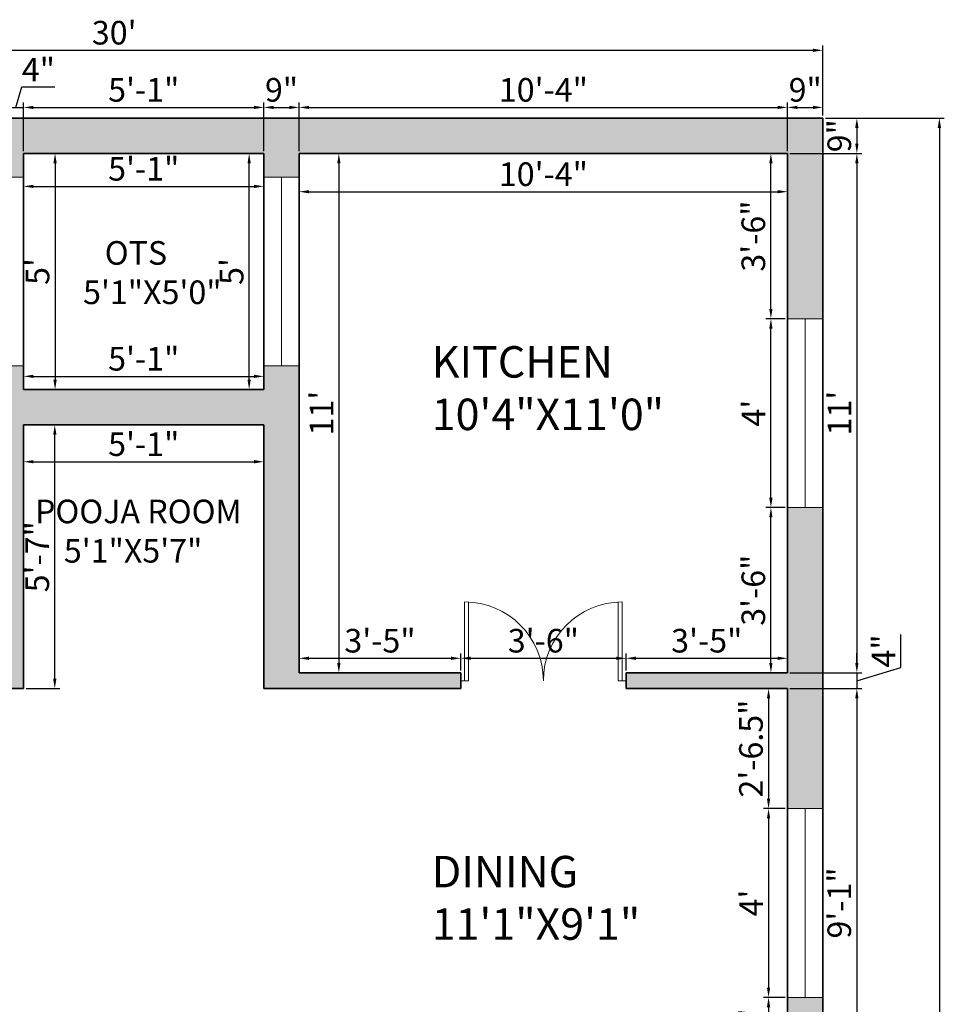
# Model space of a CAD drawing. Units: inches. Extents: x 3592 to 4861, y 1650 to 2243.
# Tile 30 of 30: x 4622 to 4857, y 1940 to 2190. Entities that reach past the tile are written whole.
import ezdxf

# ---------------------------------------------------------------- set-up
doc = ezdxf.new("R2010")
doc.units = ezdxf.units.IN
for name, color, linetype, lineweight in [('A-ANNO-DIMS', 2, 'Continuous', 13), ('A-AREA-IDEN', 7, 'Continuous', 18), ('A-DOOR', 3, 'Continuous', 20), ('A-GLAZ', 4, 'Continuous', 18), ('A-WALL', 7, 'Continuous', 35)]:
    doc.layers.add(name, color=color, linetype=linetype, lineweight=lineweight)
doc.layers.add('A-WALL-PATT', color=252, linetype='Continuous', lineweight=13, true_color=0x939598)
doc.styles.get("Standard").update_dxf_attribs({"font": 'arial.ttf'})
doc.dimstyles.new('ISO-25', dxfattribs={"dimtxt": 9, "dimasz": 2.5, "dimexe": 1.25, "dimexo": 0.625, "dimtad": 1, "dimlunit": 3, "dimtxsty": 'Standard', "dimcen": 2.5, "dimadec": 0, "dimazin": 0, "dimtfac": 1, "dimtmove": 0, "dimatfit": 3, "dimfxl": 1, "dimarcsym": 0})

# ---------------------------------------------------------------- blocks, each defined once
blk = doc.blocks.new('MD')
for p, q in [((3665.34, 1831.69), (3665.34, 1851.69)), ((3666.34, 1831.69), (3666.34, 1851.69)), ((3704.34, 1831.69), (3704.34, 1851.69)), ((3705.34, 1831.69), (3705.34, 1851.69)), ((3664.34, 1831.69), (3666.34, 1831.69)), ((3706.34, 1831.69), (3704.34, 1831.69))]:
    blk.add_line(p, q)
for centre, start, end in [((3665.34, 1831.69), 0, 90), ((3705.34, 1831.69), 90, 180)]:
    blk.add_arc(centre, 20, start, end)
blk = doc.blocks.new('*D50')
at = {"layer": 'A-ANNO-DIMS', "color": 0, "lineweight": -2, "transparency": 16777216}
for p, q in [((4623.25, 2155.59), (4623.25, 2146.6)), ((4684.25, 2155.59), (4684.25, 2146.6)), ((4625.75, 2147.85), (4681.75, 2147.85))]:
    blk.add_line(p, q, dxfattribs=at)
at = {"layer": 'A-ANNO-DIMS', "color": 0, "transparency": 16777216}
for points in [[(4625.75, 2148.27), (4625.75, 2147.43), (4623.25, 2147.85)], [(4681.75, 2148.27), (4681.75, 2147.43), (4684.25, 2147.85)]]:
    blk.add_solid(points, dxfattribs=at)
at = {"layer": 'Defpoints', "color": 0, "transparency": 16777216}
for p in [(4623.25, 2156.22), (4684.25, 2156.22), (4684.25, 2147.85)]:
    blk.add_point(p, dxfattribs=at)
at = {"layer": 'A-ANNO-DIMS', "color": 0, "transparency": 16777216, "insert": (4653.75, 2151.54), "char_height": 6, "attachment_point": 5}
blk.add_mtext('5\'-1"', dxfattribs=at)
blk = doc.blocks.new('*D51')
at = {"layer": 'A-ANNO-DIMS', "color": 0, "lineweight": -2, "transparency": 16777216}
for p, q in [((4623.87, 2156.22), (4632.48, 2156.22)), ((4631.23, 2153.72), (4631.23, 2098.72)), ((4623.87, 2096.22), (4632.48, 2096.22))]:
    blk.add_line(p, q, dxfattribs=at)
at = {"layer": 'A-ANNO-DIMS', "color": 0, "transparency": 16777216}
for points in [[(4630.81, 2153.72), (4631.65, 2153.72), (4631.23, 2156.22)], [(4630.81, 2098.72), (4631.65, 2098.72), (4631.23, 2096.22)]]:
    blk.add_solid(points, dxfattribs=at)
at = {"layer": 'Defpoints', "color": 0, "transparency": 16777216}
for p in [(4623.25, 2156.22), (4623.25, 2096.22), (4631.23, 2096.22)]:
    blk.add_point(p, dxfattribs=at)
at = {"layer": 'A-ANNO-DIMS', "color": 0, "transparency": 16777216, "insert": (4627.55, 2126.22), "char_height": 6, "attachment_point": 5, "rotation": 90}
blk.add_mtext("5'", dxfattribs=at)
blk = doc.blocks.new('*D52')
at = {"layer": 'A-ANNO-DIMS', "color": 0, "lineweight": -2, "transparency": 16777216}
for p, q in [((4623.25, 2096.84), (4623.25, 2100.82)), ((4625.75, 2099.57), (4681.75, 2099.57)), ((4684.25, 2096.84), (4684.25, 2100.82))]:
    blk.add_line(p, q, dxfattribs=at)
at = {"layer": 'A-ANNO-DIMS', "color": 0, "transparency": 16777216}
for points in [[(4625.75, 2099.99), (4625.75, 2099.15), (4623.25, 2099.57)], [(4681.75, 2099.99), (4681.75, 2099.15), (4684.25, 2099.57)]]:
    blk.add_solid(points, dxfattribs=at)
at = {"layer": 'Defpoints', "color": 0, "transparency": 16777216}
for p in [(4684.25, 2099.57), (4623.25, 2096.22), (4684.25, 2096.22)]:
    blk.add_point(p, dxfattribs=at)
at = {"layer": 'A-ANNO-DIMS', "color": 0, "transparency": 16777216, "insert": (4653.75, 2103.26), "char_height": 6, "attachment_point": 5}
blk.add_mtext('5\'-1"', dxfattribs=at)
blk = doc.blocks.new('*D53')
at = {"layer": 'A-ANNO-DIMS', "color": 0, "lineweight": -2, "transparency": 16777216}
for p, q in [((4683.62, 2156.22), (4679.27, 2156.22)), ((4680.52, 2098.72), (4680.52, 2153.72)), ((4683.62, 2096.22), (4679.27, 2096.22))]:
    blk.add_line(p, q, dxfattribs=at)
at = {"layer": 'A-ANNO-DIMS', "color": 0, "transparency": 16777216}
for points in [[(4680.11, 2153.72), (4680.94, 2153.72), (4680.52, 2156.22)], [(4680.11, 2098.72), (4680.94, 2098.72), (4680.52, 2096.22)]]:
    blk.add_solid(points, dxfattribs=at)
at = {"layer": 'Defpoints', "color": 0, "transparency": 16777216}
for p in [(4680.52, 2156.22), (4684.25, 2156.22), (4684.25, 2096.22)]:
    blk.add_point(p, dxfattribs=at)
at = {"layer": 'A-ANNO-DIMS', "color": 0, "transparency": 16777216, "insert": (4676.85, 2126.22), "char_height": 6, "attachment_point": 5, "rotation": 90}
blk.add_mtext("5'", dxfattribs=at)
blk = doc.blocks.new('*D54')
at = {"layer": 'A-ANNO-DIMS', "color": 0, "lineweight": -2, "transparency": 16777216}
for p, q in [((4693.87, 2156.22), (4704.56, 2156.22)), ((4703.31, 2153.72), (4703.31, 2026.72)), ((4693.87, 2024.22), (4704.56, 2024.22))]:
    blk.add_line(p, q, dxfattribs=at)
at = {"layer": 'A-ANNO-DIMS', "color": 0, "transparency": 16777216}
for points in [[(4702.89, 2153.72), (4703.72, 2153.72), (4703.31, 2156.22)], [(4702.89, 2026.72), (4703.72, 2026.72), (4703.31, 2024.22)]]:
    blk.add_solid(points, dxfattribs=at)
at = {"layer": 'Defpoints', "color": 0, "transparency": 16777216}
for p in [(4693.25, 2156.22), (4693.25, 2024.22), (4703.31, 2024.22)]:
    blk.add_point(p, dxfattribs=at)
at = {"layer": 'A-ANNO-DIMS', "color": 0, "transparency": 16777216, "insert": (4699.67, 2090.22), "char_height": 6, "attachment_point": 5, "rotation": 90}
blk.add_mtext("11'", dxfattribs=at)
blk = doc.blocks.new('*D55')
at = {"layer": 'A-ANNO-DIMS', "color": 0, "lineweight": -2, "transparency": 16777216}
for p, q in [((4693.25, 2155.59), (4693.25, 2145.25)), ((4817.25, 2155.59), (4817.25, 2145.25)), ((4695.75, 2146.5), (4814.75, 2146.5))]:
    blk.add_line(p, q, dxfattribs=at)
at = {"layer": 'A-ANNO-DIMS', "color": 0, "transparency": 16777216}
for points in [[(4695.75, 2146.91), (4695.75, 2146.08), (4693.25, 2146.5)], [(4814.75, 2146.91), (4814.75, 2146.08), (4817.25, 2146.5)]]:
    blk.add_solid(points, dxfattribs=at)
at = {"layer": 'Defpoints', "color": 0, "transparency": 16777216}
for p in [(4693.25, 2156.22), (4817.25, 2156.22), (4817.25, 2146.5)]:
    blk.add_point(p, dxfattribs=at)
at = {"layer": 'A-ANNO-DIMS', "color": 0, "transparency": 16777216, "insert": (4755.25, 2150.18), "char_height": 6, "attachment_point": 5}
blk.add_mtext('10\'-4"', dxfattribs=at)
blk = doc.blocks.new('*D59')
at = {"layer": 'A-ANNO-DIMS', "color": 0, "lineweight": -2, "transparency": 16777216}
for p, q in [((4623.87, 2087.22), (4632.41, 2087.22)), ((4631.16, 2022.72), (4631.16, 2084.72)), ((4623.87, 2020.22), (4632.41, 2020.22))]:
    blk.add_line(p, q, dxfattribs=at)
at = {"layer": 'A-ANNO-DIMS', "color": 0, "transparency": 16777216}
for points in [[(4630.74, 2084.72), (4631.58, 2084.72), (4631.16, 2087.22)], [(4630.74, 2022.72), (4631.58, 2022.72), (4631.16, 2020.22)]]:
    blk.add_solid(points, dxfattribs=at)
at = {"layer": 'Defpoints', "color": 0, "transparency": 16777216}
for p in [(4623.25, 2087.22), (4631.16, 2087.22), (4623.25, 2020.22)]:
    blk.add_point(p, dxfattribs=at)
at = {"layer": 'A-ANNO-DIMS', "color": 0, "transparency": 16777216, "insert": (4627.48, 2053.72), "char_height": 6, "attachment_point": 5, "rotation": 90}
blk.add_mtext('5\'-7"', dxfattribs=at)
blk = doc.blocks.new('*D60')
at = {"layer": 'A-ANNO-DIMS', "color": 0, "lineweight": -2, "transparency": 16777216}
for p, q in [((4623.25, 2086.59), (4623.25, 2076.62)), ((4684.25, 2086.59), (4684.25, 2076.62)), ((4625.75, 2077.87), (4681.75, 2077.87))]:
    blk.add_line(p, q, dxfattribs=at)
at = {"layer": 'A-ANNO-DIMS', "color": 0, "transparency": 16777216}
for points in [[(4625.75, 2078.29), (4625.75, 2077.45), (4623.25, 2077.87)], [(4681.75, 2078.29), (4681.75, 2077.45), (4684.25, 2077.87)]]:
    blk.add_solid(points, dxfattribs=at)
at = {"layer": 'Defpoints', "color": 0, "transparency": 16777216}
for p in [(4623.25, 2087.22), (4684.25, 2087.22), (4684.25, 2077.87)]:
    blk.add_point(p, dxfattribs=at)
at = {"layer": 'A-ANNO-DIMS', "color": 0, "transparency": 16777216, "insert": (4653.75, 2081.56), "char_height": 6, "attachment_point": 5}
blk.add_mtext('5\'-1"', dxfattribs=at)
blk = doc.blocks.new('*D61')
at = {"layer": 'A-ANNO-DIMS', "color": 0, "lineweight": -2, "transparency": 16777216}
for p, q in [((4693.25, 2024.84), (4693.25, 2029.16)), ((4695.75, 2027.91), (4731.75, 2027.91)), ((4734.25, 2024.84), (4734.25, 2029.16))]:
    blk.add_line(p, q, dxfattribs=at)
at = {"layer": 'A-ANNO-DIMS', "color": 0, "transparency": 16777216}
for points in [[(4695.75, 2028.33), (4695.75, 2027.49), (4693.25, 2027.91)], [(4731.75, 2028.33), (4731.75, 2027.49), (4734.25, 2027.91)]]:
    blk.add_solid(points, dxfattribs=at)
at = {"layer": 'Defpoints', "color": 0, "transparency": 16777216}
for p in [(4734.25, 2027.91), (4693.25, 2024.22), (4734.25, 2024.22)]:
    blk.add_point(p, dxfattribs=at)
at = {"layer": 'A-ANNO-DIMS', "color": 0, "transparency": 16777216, "insert": (4713.75, 2031.6), "char_height": 6, "attachment_point": 5}
blk.add_mtext('3\'-5"', dxfattribs=at)
blk = doc.blocks.new('*D62')
at = {"layer": 'A-ANNO-DIMS', "color": 0, "lineweight": -2, "transparency": 16777216}
for p, q in [((4734.25, 2024.84), (4734.25, 2029.16)), ((4736.75, 2027.91), (4773.75, 2027.91)), ((4776.25, 2024.84), (4776.25, 2029.16))]:
    blk.add_line(p, q, dxfattribs=at)
at = {"layer": 'A-ANNO-DIMS', "color": 0, "transparency": 16777216}
for points in [[(4736.75, 2028.33), (4736.75, 2027.49), (4734.25, 2027.91)], [(4773.75, 2028.33), (4773.75, 2027.49), (4776.25, 2027.91)]]:
    blk.add_solid(points, dxfattribs=at)
at = {"layer": 'Defpoints', "color": 0, "transparency": 16777216}
for p in [(4776.25, 2027.91), (4734.25, 2024.22), (4776.25, 2024.22)]:
    blk.add_point(p, dxfattribs=at)
at = {"layer": 'A-ANNO-DIMS', "color": 0, "transparency": 16777216, "insert": (4755.25, 2031.6), "char_height": 6, "attachment_point": 5}
blk.add_mtext('3\'-6"', dxfattribs=at)
blk = doc.blocks.new('*D63')
at = {"layer": 'A-ANNO-DIMS', "color": 0, "lineweight": -2, "transparency": 16777216}
for p, q in [((4776.25, 2024.84), (4776.25, 2029.16)), ((4778.75, 2027.91), (4814.75, 2027.91)), ((4817.25, 2024.84), (4817.25, 2029.16))]:
    blk.add_line(p, q, dxfattribs=at)
at = {"layer": 'A-ANNO-DIMS', "color": 0, "transparency": 16777216}
for points in [[(4778.75, 2028.33), (4778.75, 2027.49), (4776.25, 2027.91)], [(4814.75, 2028.33), (4814.75, 2027.49), (4817.25, 2027.91)]]:
    blk.add_solid(points, dxfattribs=at)
at = {"layer": 'Defpoints', "color": 0, "transparency": 16777216}
for p in [(4817.25, 2027.91), (4776.25, 2024.22), (4817.25, 2024.22)]:
    blk.add_point(p, dxfattribs=at)
at = {"layer": 'A-ANNO-DIMS', "color": 0, "transparency": 16777216, "insert": (4796.75, 2031.6), "char_height": 6, "attachment_point": 5}
blk.add_mtext('3\'-5"', dxfattribs=at)
blk = doc.blocks.new('*D64')
at = {"layer": 'A-ANNO-DIMS', "color": 0, "lineweight": -2, "transparency": 16777216}
for p, q in [((4816.62, 2066.22), (4811.79, 2066.22)), ((4813.04, 2026.72), (4813.04, 2063.72)), ((4816.62, 2024.22), (4811.79, 2024.22))]:
    blk.add_line(p, q, dxfattribs=at)
at = {"layer": 'A-ANNO-DIMS', "color": 0, "transparency": 16777216}
for points in [[(4812.62, 2063.72), (4813.45, 2063.72), (4813.04, 2066.22)], [(4812.62, 2026.72), (4813.45, 2026.72), (4813.04, 2024.22)]]:
    blk.add_solid(points, dxfattribs=at)
at = {"layer": 'Defpoints', "color": 0, "transparency": 16777216}
for p in [(4813.04, 2066.22), (4817.25, 2066.22), (4817.25, 2024.22)]:
    blk.add_point(p, dxfattribs=at)
at = {"layer": 'A-ANNO-DIMS', "color": 0, "transparency": 16777216, "insert": (4809.35, 2045.22), "char_height": 6, "attachment_point": 5, "rotation": 90}
blk.add_mtext('3\'-6"', dxfattribs=at)
blk = doc.blocks.new('*D65')
at = {"layer": 'A-ANNO-DIMS', "color": 0, "lineweight": -2, "transparency": 16777216}
for p, q in [((4816.62, 2114.22), (4811.79, 2114.22)), ((4813.04, 2068.72), (4813.04, 2111.72)), ((4816.62, 2066.22), (4811.79, 2066.22))]:
    blk.add_line(p, q, dxfattribs=at)
at = {"layer": 'A-ANNO-DIMS', "color": 0, "transparency": 16777216}
for points in [[(4812.62, 2111.72), (4813.45, 2111.72), (4813.04, 2114.22)], [(4812.62, 2068.72), (4813.45, 2068.72), (4813.04, 2066.22)]]:
    blk.add_solid(points, dxfattribs=at)
at = {"layer": 'Defpoints', "color": 0, "transparency": 16777216}
for p in [(4813.04, 2114.22), (4817.25, 2114.22), (4817.25, 2066.22)]:
    blk.add_point(p, dxfattribs=at)
at = {"layer": 'A-ANNO-DIMS', "color": 0, "transparency": 16777216, "insert": (4809.41, 2090.22), "char_height": 6, "attachment_point": 5, "rotation": 90}
blk.add_mtext("4'", dxfattribs=at)
blk = doc.blocks.new('*D66')
at = {"layer": 'A-ANNO-DIMS', "color": 0, "lineweight": -2, "transparency": 16777216}
for p, q in [((4816.62, 2156.22), (4811.79, 2156.22)), ((4813.04, 2116.72), (4813.04, 2153.72)), ((4816.62, 2114.22), (4811.79, 2114.22))]:
    blk.add_line(p, q, dxfattribs=at)
at = {"layer": 'A-ANNO-DIMS', "color": 0, "transparency": 16777216}
for points in [[(4812.62, 2153.72), (4813.45, 2153.72), (4813.04, 2156.22)], [(4812.62, 2116.72), (4813.45, 2116.72), (4813.04, 2114.22)]]:
    blk.add_solid(points, dxfattribs=at)
at = {"layer": 'Defpoints', "color": 0, "transparency": 16777216}
for p in [(4813.04, 2156.22), (4817.25, 2156.22), (4817.25, 2114.22)]:
    blk.add_point(p, dxfattribs=at)
at = {"layer": 'A-ANNO-DIMS', "color": 0, "transparency": 16777216, "insert": (4809.35, 2135.22), "char_height": 6, "attachment_point": 5, "rotation": 90}
blk.add_mtext('3\'-6"', dxfattribs=at)
blk = doc.blocks.new('*D67')
at = {"layer": 'A-ANNO-DIMS', "color": 0, "lineweight": -2, "transparency": 16777216}
for p, q in [((4816.62, 2020.22), (4811.19, 2020.22)), ((4812.44, 2017.72), (4812.44, 1992.22)), ((4816.62, 1989.72), (4811.19, 1989.72))]:
    blk.add_line(p, q, dxfattribs=at)
at = {"layer": 'A-ANNO-DIMS', "color": 0, "transparency": 16777216}
for points in [[(4812.03, 2017.72), (4812.86, 2017.72), (4812.44, 2020.22)], [(4812.03, 1992.22), (4812.86, 1992.22), (4812.44, 1989.72)]]:
    blk.add_solid(points, dxfattribs=at)
at = {"layer": 'Defpoints', "color": 0, "transparency": 16777216}
for p in [(4817.25, 2020.22), (4812.44, 1989.72), (4817.25, 1989.72)]:
    blk.add_point(p, dxfattribs=at)
at = {"layer": 'A-ANNO-DIMS', "color": 0, "transparency": 16777216, "insert": (4808.75, 2004.97), "char_height": 6, "attachment_point": 5, "rotation": 90}
blk.add_mtext('2\'-6.5"', dxfattribs=at)
blk = doc.blocks.new('*D68')
at = {"layer": 'A-ANNO-DIMS', "color": 0, "lineweight": -2, "transparency": 16777216}
for p, q in [((4816.62, 1989.72), (4811.19, 1989.72)), ((4812.44, 1987.22), (4812.44, 1944.22)), ((4816.62, 1941.72), (4811.19, 1941.72))]:
    blk.add_line(p, q, dxfattribs=at)
at = {"layer": 'A-ANNO-DIMS', "color": 0, "transparency": 16777216}
for points in [[(4812.03, 1987.22), (4812.86, 1987.22), (4812.44, 1989.72)], [(4812.03, 1944.22), (4812.86, 1944.22), (4812.44, 1941.72)]]:
    blk.add_solid(points, dxfattribs=at)
at = {"layer": 'Defpoints', "color": 0, "transparency": 16777216}
for p in [(4817.25, 1989.72), (4812.44, 1941.72), (4817.25, 1941.72)]:
    blk.add_point(p, dxfattribs=at)
at = {"layer": 'A-ANNO-DIMS', "color": 0, "transparency": 16777216, "insert": (4808.82, 1965.72), "char_height": 6, "attachment_point": 5, "rotation": 90}
blk.add_mtext("4'", dxfattribs=at)
blk = doc.blocks.new('*D69')
at = {"layer": 'A-ANNO-DIMS', "color": 0, "lineweight": -2, "transparency": 16777216}
for p, q in [((4816.62, 1941.72), (4811.19, 1941.72)), ((4812.44, 1939.22), (4812.44, 1913.72)), ((4816.62, 1911.22), (4811.19, 1911.22))]:
    blk.add_line(p, q, dxfattribs=at)
at = {"layer": 'A-ANNO-DIMS', "color": 0, "transparency": 16777216}
for points in [[(4812.03, 1939.22), (4812.86, 1939.22), (4812.44, 1941.72)], [(4812.03, 1913.72), (4812.86, 1913.72), (4812.44, 1911.22)]]:
    blk.add_solid(points, dxfattribs=at)
at = {"layer": 'Defpoints', "color": 0, "transparency": 16777216}
for p in [(4817.25, 1941.72), (4812.44, 1911.22), (4817.25, 1911.22)]:
    blk.add_point(p, dxfattribs=at)
at = {"layer": 'A-ANNO-DIMS', "color": 0, "transparency": 16777216, "insert": (4808.75, 1926.47), "char_height": 6, "attachment_point": 5, "rotation": 90}
blk.add_mtext('2\'-6.5"', dxfattribs=at)
blk = doc.blocks.new('*D113')
at = {"layer": 'A-ANNO-DIMS', "color": 0, "lineweight": -2, "transparency": 16777216}
for p, q in [((4621.25, 2167.92), (4622.81, 2173.11)), ((4622.81, 2173.11), (4631.19, 2173.11)), ((4616.75, 2167.92), (4614.25, 2167.92)), ((4619.25, 2156.84), (4619.25, 2169.17)), ((4619.25, 2167.92), (4623.25, 2167.92)), ((4619.25, 2167.92), (4623.25, 2167.92)), ((4623.25, 2156.84), (4623.25, 2169.17)), ((4625.75, 2167.92), (4628.25, 2167.92))]:
    blk.add_line(p, q, dxfattribs=at)
at = {"layer": 'A-ANNO-DIMS', "color": 0, "transparency": 16777216}
for points in [[(4616.75, 2168.33), (4616.75, 2167.5), (4619.25, 2167.92)], [(4625.75, 2168.33), (4625.75, 2167.5), (4623.25, 2167.92)]]:
    blk.add_solid(points, dxfattribs=at)
at = {"layer": 'Defpoints', "color": 0, "transparency": 16777216}
for p in [(4623.25, 2167.92), (4619.25, 2156.22), (4623.25, 2156.22)]:
    blk.add_point(p, dxfattribs=at)
at = {"layer": 'A-ANNO-DIMS', "color": 0, "transparency": 16777216, "insert": (4627, 2176.73), "char_height": 6, "attachment_point": 5}
blk.add_mtext('4"', dxfattribs=at)
blk = doc.blocks.new('*D114')
at = {"layer": 'A-ANNO-DIMS', "color": 0, "lineweight": -2, "transparency": 16777216}
for p, q in [((4623.25, 2156.84), (4623.25, 2169.17)), ((4625.75, 2167.92), (4681.75, 2167.92)), ((4684.25, 2156.84), (4684.25, 2169.17))]:
    blk.add_line(p, q, dxfattribs=at)
at = {"layer": 'A-ANNO-DIMS', "color": 0, "transparency": 16777216}
for points in [[(4625.75, 2168.33), (4625.75, 2167.5), (4623.25, 2167.92)], [(4681.75, 2168.33), (4681.75, 2167.5), (4684.25, 2167.92)]]:
    blk.add_solid(points, dxfattribs=at)
at = {"layer": 'Defpoints', "color": 0, "transparency": 16777216}
for p in [(4684.25, 2167.92), (4623.25, 2156.22), (4684.25, 2156.22)]:
    blk.add_point(p, dxfattribs=at)
at = {"layer": 'A-ANNO-DIMS', "color": 0, "transparency": 16777216, "insert": (4653.75, 2171.61), "char_height": 6, "attachment_point": 5}
blk.add_mtext('5\'-1"', dxfattribs=at)
blk = doc.blocks.new('*D115')
at = {"layer": 'A-ANNO-DIMS', "color": 0, "lineweight": -2, "transparency": 16777216}
for p, q in [((4684.25, 2156.84), (4684.25, 2169.17)), ((4686.75, 2167.92), (4690.75, 2167.92)), ((4693.25, 2156.84), (4693.25, 2169.17))]:
    blk.add_line(p, q, dxfattribs=at)
at = {"layer": 'A-ANNO-DIMS', "color": 0, "transparency": 16777216}
for points in [[(4686.75, 2168.33), (4686.75, 2167.5), (4684.25, 2167.92)], [(4690.75, 2168.33), (4690.75, 2167.5), (4693.25, 2167.92)]]:
    blk.add_solid(points, dxfattribs=at)
at = {"layer": 'Defpoints', "color": 0, "transparency": 16777216}
for p in [(4693.25, 2167.92), (4684.25, 2156.22), (4693.25, 2156.22)]:
    blk.add_point(p, dxfattribs=at)
at = {"layer": 'A-ANNO-DIMS', "color": 0, "transparency": 16777216, "insert": (4688.75, 2171.61), "char_height": 6, "attachment_point": 5}
blk.add_mtext('9"', dxfattribs=at)
blk = doc.blocks.new('*D116')
at = {"layer": 'A-ANNO-DIMS', "color": 0, "lineweight": -2, "transparency": 16777216}
for p, q in [((4693.25, 2156.84), (4693.25, 2169.17)), ((4695.75, 2167.92), (4814.75, 2167.92)), ((4817.25, 2156.84), (4817.25, 2169.17))]:
    blk.add_line(p, q, dxfattribs=at)
at = {"layer": 'A-ANNO-DIMS', "color": 0, "transparency": 16777216}
for points in [[(4695.75, 2168.33), (4695.75, 2167.5), (4693.25, 2167.92)], [(4814.75, 2168.33), (4814.75, 2167.5), (4817.25, 2167.92)]]:
    blk.add_solid(points, dxfattribs=at)
at = {"layer": 'Defpoints', "color": 0, "transparency": 16777216}
for p in [(4817.25, 2167.92), (4693.25, 2156.22), (4817.25, 2156.22)]:
    blk.add_point(p, dxfattribs=at)
at = {"layer": 'A-ANNO-DIMS', "color": 0, "transparency": 16777216, "insert": (4755.25, 2171.61), "char_height": 6, "attachment_point": 5}
blk.add_mtext('10\'-4"', dxfattribs=at)
blk = doc.blocks.new('*D117')
at = {"layer": 'A-ANNO-DIMS', "color": 0, "lineweight": -2, "transparency": 16777216}
for p, q in [((4817.25, 2156.84), (4817.25, 2169.17)), ((4819.75, 2167.92), (4823.75, 2167.92)), ((4826.25, 2165.84), (4826.25, 2169.17))]:
    blk.add_line(p, q, dxfattribs=at)
at = {"layer": 'A-ANNO-DIMS', "color": 0, "transparency": 16777216}
for points in [[(4819.75, 2168.33), (4819.75, 2167.5), (4817.25, 2167.92)], [(4823.75, 2168.33), (4823.75, 2167.5), (4826.25, 2167.92)]]:
    blk.add_solid(points, dxfattribs=at)
at = {"layer": 'Defpoints', "color": 0, "transparency": 16777216}
for p in [(4826.25, 2167.92), (4826.25, 2165.22), (4817.25, 2156.22)]:
    blk.add_point(p, dxfattribs=at)
at = {"layer": 'A-ANNO-DIMS', "color": 0, "transparency": 16777216, "insert": (4821.75, 2171.61), "char_height": 6, "attachment_point": 5}
blk.add_mtext('9"', dxfattribs=at)
blk = doc.blocks.new('*D118')
at = {"layer": 'A-ANNO-DIMS', "color": 0, "lineweight": -2, "transparency": 16777216}
for p, q in [((4826.87, 2165.22), (4836.12, 2165.22)), ((4834.87, 2162.72), (4834.87, 2158.72)), ((4817.87, 2156.22), (4836.12, 2156.22))]:
    blk.add_line(p, q, dxfattribs=at)
at = {"layer": 'A-ANNO-DIMS', "color": 0, "transparency": 16777216}
for points in [[(4834.45, 2162.72), (4835.29, 2162.72), (4834.87, 2165.22)], [(4834.45, 2158.72), (4835.29, 2158.72), (4834.87, 2156.22)]]:
    blk.add_solid(points, dxfattribs=at)
at = {"layer": 'Defpoints', "color": 0, "transparency": 16777216}
for p in [(4826.25, 2165.22), (4817.25, 2156.22), (4834.87, 2156.22)]:
    blk.add_point(p, dxfattribs=at)
at = {"layer": 'A-ANNO-DIMS', "color": 0, "transparency": 16777216, "insert": (4831.18, 2160.72), "char_height": 6, "attachment_point": 5, "rotation": 90}
blk.add_mtext('9"', dxfattribs=at)
blk = doc.blocks.new('*D119')
at = {"layer": 'A-ANNO-DIMS', "color": 0, "lineweight": -2, "transparency": 16777216}
for p, q in [((4817.87, 2156.22), (4836.12, 2156.22)), ((4834.87, 2153.72), (4834.87, 2026.72)), ((4817.87, 2024.22), (4836.12, 2024.22))]:
    blk.add_line(p, q, dxfattribs=at)
at = {"layer": 'A-ANNO-DIMS', "color": 0, "transparency": 16777216}
for points in [[(4834.45, 2153.72), (4835.29, 2153.72), (4834.87, 2156.22)], [(4834.45, 2026.72), (4835.29, 2026.72), (4834.87, 2024.22)]]:
    blk.add_solid(points, dxfattribs=at)
at = {"layer": 'Defpoints', "color": 0, "transparency": 16777216}
for p in [(4817.25, 2156.22), (4817.25, 2024.22), (4834.87, 2024.22)]:
    blk.add_point(p, dxfattribs=at)
at = {"layer": 'A-ANNO-DIMS', "color": 0, "transparency": 16777216, "insert": (4831.23, 2090.22), "char_height": 6, "attachment_point": 5, "rotation": 90}
blk.add_mtext("11'", dxfattribs=at)
blk = doc.blocks.new('*D120')
at = {"layer": 'A-ANNO-DIMS', "color": 0, "lineweight": -2, "transparency": 16777216}
for p, q in [((4846.06, 2025.58), (4846.06, 2033.96)), ((4834.87, 2026.72), (4834.87, 2029.22)), ((4834.87, 2022.22), (4846.06, 2025.58)), ((4817.87, 2024.22), (4836.12, 2024.22)), ((4834.87, 2024.22), (4834.87, 2020.22)), ((4834.87, 2024.22), (4834.87, 2020.22)), ((4817.87, 2020.22), (4836.12, 2020.22)), ((4834.87, 2017.72), (4834.87, 2015.22))]:
    blk.add_line(p, q, dxfattribs=at)
at = {"layer": 'A-ANNO-DIMS', "color": 0, "transparency": 16777216}
for points in [[(4834.45, 2026.72), (4835.29, 2026.72), (4834.87, 2024.22)], [(4834.45, 2017.72), (4835.29, 2017.72), (4834.87, 2020.22)]]:
    blk.add_solid(points, dxfattribs=at)
at = {"layer": 'Defpoints', "color": 0, "transparency": 16777216}
for p in [(4817.25, 2024.22), (4817.25, 2020.22), (4834.87, 2020.22)]:
    blk.add_point(p, dxfattribs=at)
at = {"layer": 'A-ANNO-DIMS', "color": 0, "transparency": 16777216, "insert": (4842.43, 2029.77), "char_height": 6, "attachment_point": 5, "rotation": 90}
blk.add_mtext('4"', dxfattribs=at)
blk = doc.blocks.new('*D121')
at = {"layer": 'A-ANNO-DIMS', "color": 0, "lineweight": -2, "transparency": 16777216}
for p, q in [((4817.87, 2020.22), (4836.12, 2020.22)), ((4834.87, 2017.72), (4834.87, 1913.72)), ((4817.87, 1911.22), (4836.12, 1911.22))]:
    blk.add_line(p, q, dxfattribs=at)
at = {"layer": 'A-ANNO-DIMS', "color": 0, "transparency": 16777216}
for points in [[(4834.45, 2017.72), (4835.29, 2017.72), (4834.87, 2020.22)], [(4834.45, 1913.72), (4835.29, 1913.72), (4834.87, 1911.22)]]:
    blk.add_solid(points, dxfattribs=at)
at = {"layer": 'Defpoints', "color": 0, "transparency": 16777216}
for p in [(4817.25, 2020.22), (4817.25, 1911.22), (4834.87, 1911.22)]:
    blk.add_point(p, dxfattribs=at)
at = {"layer": 'A-ANNO-DIMS', "color": 0, "transparency": 16777216, "insert": (4831.18, 1965.72), "char_height": 6, "attachment_point": 5, "rotation": 90}
blk.add_mtext('9\'-1"', dxfattribs=at)
blk = doc.blocks.new('*D132')
at = {"layer": 'A-ANNO-DIMS', "color": 0, "lineweight": -2, "transparency": 16777216}
for p, q in [((4466.25, 2165.84), (4466.25, 2183.69)), ((4468.75, 2182.44), (4823.75, 2182.44)), ((4826.25, 2165.84), (4826.25, 2183.69))]:
    blk.add_line(p, q, dxfattribs=at)
at = {"layer": 'A-ANNO-DIMS', "color": 0, "transparency": 16777216}
for points in [[(4468.75, 2182.85), (4468.75, 2182.02), (4466.25, 2182.44)], [(4823.75, 2182.85), (4823.75, 2182.02), (4826.25, 2182.44)]]:
    blk.add_solid(points, dxfattribs=at)
at = {"layer": 'Defpoints', "color": 0, "transparency": 16777216}
for p in [(4826.25, 2182.44), (4466.25, 2165.22), (4826.25, 2165.22)]:
    blk.add_point(p, dxfattribs=at)
at = {"layer": 'A-ANNO-DIMS', "color": 0, "transparency": 16777216, "insert": (4646.25, 2186.13), "char_height": 6, "attachment_point": 5}
blk.add_mtext("30'", dxfattribs=at)
blk = doc.blocks.new('*D133')
at = {"layer": 'A-ANNO-DIMS', "color": 0, "lineweight": -2, "transparency": 16777216}
for p, q in [((4826.87, 2165.22), (4857.08, 2165.22)), ((4855.83, 2162.72), (4855.83, 1687.72)), ((4826.87, 1685.22), (4857.08, 1685.22))]:
    blk.add_line(p, q, dxfattribs=at)
at = {"layer": 'A-ANNO-DIMS', "color": 0, "transparency": 16777216}
for points in [[(4855.41, 2162.72), (4856.24, 2162.72), (4855.83, 2165.22)], [(4855.41, 1687.72), (4856.24, 1687.72), (4855.83, 1685.22)]]:
    blk.add_solid(points, dxfattribs=at)
at = {"layer": 'Defpoints', "color": 0, "transparency": 16777216}
for p in [(4826.25, 2165.22), (4826.25, 1685.22), (4855.83, 1685.22)]:
    blk.add_point(p, dxfattribs=at)
at = {"layer": 'A-ANNO-DIMS', "color": 0, "transparency": 16777216, "insert": (4852.14, 1925.22), "char_height": 6, "attachment_point": 5, "rotation": 90}
blk.add_mtext("40'", dxfattribs=at)

msp = doc.modelspace()

# ---------------------------------------------------------------- hatches: boundary and pattern name
at = {"layer": 'A-WALL-PATT'}
h = msp.add_hatch(color=256, dxfattribs=at)
h.dxf.hatch_style = 1
h.paths.add_polyline_path([(4466.25, 2165.219), (4466.25, 1993.219), (4475.25, 1993.219), (4475.25, 2156.219), (4619.25, 2156.219), (4619.25, 2150.219), (4623.25, 2150.219), (4623.25, 2156.219), (4684.25, 2156.219), (4684.25, 2150.219), (4693.25, 2150.219), (4693.25, 2156.219), (4817.25, 2156.219), (4817.25, 2114.219), (4826.25, 2114.219), (4826.25, 2165.219)])
h.paths.add_polyline_path([(4623.25, 2096.219), (4623.25, 2102.219), (4619.25, 2102.219), (4619.25, 2020.219), (4623.25, 2020.219), (4623.25, 2087.219), (4684.25, 2087.219), (4684.25, 2020.219), (4734.25, 2020.219), (4734.25, 2024.219), (4693.25, 2024.219), (4693.25, 2102.219), (4684.25, 2102.219), (4684.25, 2096.219)], flags=17)
h.paths.add_polyline_path([(4817.25, 2024.219), (4776.25, 2024.219), (4776.25, 2020.219), (4817.25, 2020.219), (4817.25, 1989.719), (4826.25, 1989.719), (4826.25, 2066.219), (4817.25, 2066.219)])
h.paths.add_polyline_path([(4817.25, 1865.219), (4826.25, 1865.219), (4826.25, 1941.719), (4817.25, 1941.719), (4817.25, 1911.219), (4729.25, 1911.219), (4729.25, 1907.219), (4817.25, 1907.219)])
h.paths.add_polyline_path([(4826.25, 1817.219), (4817.25, 1817.219), (4817.25, 1775.219), (4693.25, 1775.219), (4693.25, 1911.219), (4684.25, 1911.219), (4684.25, 1817.219), (4648.75, 1817.219), (4648.75, 1808.219), (4684.25, 1808.219), (4684.25, 1766.219), (4817.25, 1766.219), (4817.25, 1694.219), (4684.25, 1694.219), (4684.25, 1685.219), (4826.25, 1685.219)])
h.paths.add_polyline_path([(4505.25, 1817.219), (4505.25, 1808.219), (4606.75, 1808.219), (4606.75, 1817.219)])
h.paths.add_polyline_path([(4539.25, 1856.219), (4539.25, 2020.219), (4583.25, 2020.219), (4583.25, 2024.219), (4505.25, 2024.219), (4505.25, 2020.219), (4535.25, 2020.219), (4535.25, 1942.219), (4475.25, 1942.219), (4475.25, 1969.219), (4466.25, 1969.219), (4466.25, 1911.219), (4475.25, 1911.219), (4475.25, 1938.219), (4535.25, 1938.219), (4535.25, 1860.219), (4505.25, 1860.219), (4505.25, 1856.219)])
h.paths.add_polyline_path([(4475.25, 1887.219), (4466.25, 1887.219), (4466.25, 1685.219), (4580.25, 1685.219), (4580.25, 1715.219), (4571.25, 1715.219), (4571.25, 1694.219), (4475.25, 1694.219)])
h.paths.add_polyline_path([(4571.25, 1751.219), (4580.25, 1751.219), (4580.25, 1772.219), (4571.25, 1772.219)], flags=17)

# ---------------------------------------------------------------- linework, layer by layer
at = {"layer": 'A-GLAZ'}
for p, q in [((4623.25, 2150.219), (4619.25, 2150.219)), ((4693.25, 2150.219), (4684.25, 2150.219)), ((4688.75, 2150.219), (4688.75, 2102.219)), ((4817.25, 2114.219), (4826.25, 2114.219)), ((4821.75, 2114.219), (4821.75, 2066.219)), ((4623.25, 2102.219), (4619.25, 2102.219)), ((4693.25, 2102.219), (4684.25, 2102.219)), ((4817.25, 2066.219), (4826.25, 2066.219)), ((4817.25, 1989.719), (4826.25, 1989.719)), ((4821.75, 1989.719), (4821.75, 1941.719)), ((4817.25, 1941.719), (4826.25, 1941.719))]:
    msp.add_line(p, q, dxfattribs=at)
at = {"layer": 'A-WALL'}
for p, q in [((4466.25, 2165.219), (4826.25, 2165.219)), ((4826.25, 2165.219), (4826.25, 1685.219)), ((4623.25, 2156.219), (4684.25, 2156.219)), ((4623.25, 2096.219), (4623.25, 2156.219)), ((4684.25, 2156.219), (4684.25, 2096.219)), ((4693.25, 2156.219), (4817.25, 2156.219)), ((4693.25, 2156.219), (4693.25, 2024.219)), ((4817.25, 2156.219), (4817.25, 2024.219)), ((4623.25, 2096.219), (4684.25, 2096.219)), ((4623.25, 2087.219), (4684.25, 2087.219)), ((4623.25, 2020.219), (4623.25, 2087.219)), ((4684.25, 2087.219), (4684.25, 2020.219)), ((4693.25, 2024.219), (4734.25, 2024.219)), ((4734.25, 2024.219), (4734.25, 2020.219)), ((4776.25, 2024.219), (4817.25, 2024.219)), ((4776.25, 2024.219), (4776.25, 2020.219)), ((4619.25, 2020.219), (4623.25, 2020.219)), ((4684.25, 2020.219), (4734.25, 2020.219)), ((4776.25, 2020.219), (4817.25, 2020.219)), ((4817.25, 2020.219), (4817.25, 1911.219))]:
    msp.add_line(p, q, dxfattribs=at)

# ---------------------------------------------------------------- block references
at = {"layer": 'A-DOOR'}
msp.add_blockref('MD', (1069.914, 190.53), dxfattribs=at)

# ---------------------------------------------------------------- texts
at = {"layer": 'A-AREA-IDEN', "attachment_point": 1}
for s, insert, char_height in [('   OTS\\P5\'1"X5\'0"', (4638.343, 2133.938), 6), ('KITCHEN\\P10\'4"X11\'0"', (4726.898, 2107.241), 8), ('POOJA ROOM\\P    5\'1"X5\'7"', (4626.129, 2068.232), 6), ('DINING\\P11\'1"X9\'1"', (4726.898, 1977.695), 8)]:
    msp.add_mtext_dynamic_manual_height_columns(s, width=121.44943, gutter_width=12.5, heights=[0], dxfattribs=dict(at, insert=insert, char_height=char_height))

# ---------------------------------------------------------------- dimensions: what is measured, and where the dimension line sits
at = {"layer": 'A-ANNO-DIMS'}
for base, p1, p2, override, picture, middle in [((4826.25, 2182.436), (4466.25, 2165.219), (4826.25, 2165.219), {"dimtxt": 6, "dimclrd": 0, "dimclre": 0, "dimclrt": 0}, '*D132', (4646.25, 2186.127)), ((4623.25, 2167.918), (4619.25, 2156.219), (4623.25, 2156.219), {"dimtxt": 6, "dimclrd": 0, "dimclre": 0, "dimclrt": 0, "dimtmove": 1}, '*D113', (4623.431, 2176.73)), ((4684.25, 2167.918), (4623.25, 2156.219), (4684.25, 2156.219), {"dimtxt": 6, "dimclrd": 0, "dimclre": 0, "dimclrt": 0, "dimtmove": 1}, '*D114', (4653.75, 2171.606)), ((4693.25, 2167.918), (4684.25, 2156.219), (4693.25, 2156.219), {"dimtxt": 6, "dimclrd": 0, "dimclre": 0, "dimclrt": 0, "dimtmove": 1}, '*D115', (4688.75, 2171.606)), ((4817.25, 2167.918), (4693.25, 2156.219), (4817.25, 2156.219), {"dimtxt": 6, "dimclrd": 0, "dimclre": 0, "dimclrt": 0, "dimtmove": 1}, '*D116', (4755.25, 2171.606)), ((4826.25, 2167.918), (4817.25, 2156.219), (4826.25, 2165.219), {"dimtxt": 6, "dimclrd": 0, "dimclre": 0, "dimclrt": 0, "dimtmove": 1}, '*D117', (4821.75, 2171.606)), ((4684.25, 2147.849), (4623.25, 2156.219), (4684.25, 2156.219), {"dimtxt": 6, "dimclrd": 0, "dimclre": 0, "dimclrt": 0}, '*D50', (4653.75, 2151.537)), ((4817.25, 2146.495), (4693.25, 2156.219), (4817.25, 2156.219), {"dimtxt": 6, "dimclrd": 0, "dimclre": 0, "dimclrt": 0}, '*D55', (4755.25, 2150.184)), ((4684.25, 2099.57), (4623.25, 2096.219), (4684.25, 2096.219), {"dimtxt": 6, "dimclrd": 0, "dimclre": 0, "dimclrt": 0}, '*D52', (4653.75, 2103.259)), ((4684.25, 2077.869), (4623.25, 2087.219), (4684.25, 2087.219), {"dimtxt": 6, "dimclrd": 0, "dimclre": 0, "dimclrt": 0}, '*D60', (4653.75, 2081.558)), ((4734.25, 2027.909), (4693.25, 2024.219), (4734.25, 2024.219), {"dimtxt": 6, "dimclrd": 0, "dimclre": 0, "dimclrt": 0}, '*D61', (4713.75, 2031.6)), ((4776.25, 2027.909), (4734.25, 2024.219), (4776.25, 2024.219), {"dimtxt": 6, "dimclrd": 0, "dimclre": 0, "dimclrt": 0, "dimtmove": 1}, '*D62', (4755.25, 2031.6)), ((4817.25, 2027.909), (4776.25, 2024.219), (4817.25, 2024.219), {"dimtxt": 6, "dimclrd": 0, "dimclre": 0, "dimclrt": 0, "dimtmove": 1}, '*D63', (4796.75, 2031.6))]:
    dim = msp.add_linear_dim(base=base, p1=p1, p2=p2, dimstyle='ISO-25', override=override, dxfattribs=at)
    dim.commit()
    dim.dimension.update_dxf_attribs({"geometry": picture, "text_midpoint": middle})
for base, p1, p2, override, picture, middle in [((4834.871, 2156.219), (4826.25, 2165.219), (4817.25, 2156.219), {"dimtxt": 6, "dimclrd": 0, "dimclre": 0, "dimclrt": 0}, '*D118', (4831.182, 2160.719)), ((4855.826, 1685.219), (4826.25, 2165.219), (4826.25, 1685.219), {"dimtxt": 6, "dimclrd": 0, "dimclre": 0, "dimclrt": 0}, '*D133', (4852.137, 1925.219)), ((4631.229, 2096.219), (4623.25, 2156.219), (4623.25, 2096.219), {"dimtxt": 6, "dimclrd": 0, "dimclre": 0, "dimclrt": 0}, '*D51', (4627.553, 2126.219)), ((4680.524, 2156.219), (4684.25, 2096.219), (4684.25, 2156.219), {"dimtxt": 6, "dimclrd": 0, "dimclre": 0, "dimclrt": 0}, '*D53', (4676.848, 2126.219)), ((4703.305, 2024.219), (4693.25, 2156.219), (4693.25, 2024.219), {"dimtxt": 6, "dimclrd": 0, "dimclre": 0, "dimclrt": 0}, '*D54', (4699.668, 2090.219)), ((4813.037, 2156.219), (4817.25, 2114.219), (4817.25, 2156.219), {"dimtxt": 6, "dimclrd": 0, "dimclre": 0, "dimclrt": 0, "dimtmove": 1}, '*D66', (4809.347, 2135.219)), ((4834.871, 2024.219), (4817.25, 2156.219), (4817.25, 2024.219), {"dimtxt": 6, "dimclrd": 0, "dimclre": 0, "dimclrt": 0, "dimtmove": 1}, '*D119', (4831.234, 2090.219)), ((4813.037, 2114.219), (4817.25, 2066.219), (4817.25, 2114.219), {"dimtxt": 6, "dimclrd": 0, "dimclre": 0, "dimclrt": 0, "dimtmove": 1}, '*D65', (4809.412, 2090.219)), ((4631.161, 2087.219), (4623.25, 2020.219), (4623.25, 2087.219), {"dimtxt": 6, "dimclrd": 0, "dimclre": 0, "dimclrt": 0}, '*D59', (4627.485, 2053.719)), ((4813.037, 2066.219), (4817.25, 2024.219), (4817.25, 2066.219), {"dimtxt": 6, "dimclrd": 0, "dimclre": 0, "dimclrt": 0}, '*D64', (4809.347, 2045.219)), ((4834.871, 2020.219), (4817.25, 2024.219), (4817.25, 2020.219), {"dimtxt": 6, "dimclrd": 0, "dimclre": 0, "dimclrt": 0, "dimtmove": 1}, '*D120', (4842.433, 2026.2)), ((4812.443, 1989.719), (4817.25, 2020.219), (4817.25, 1989.719), {"dimtxt": 6, "dimclrd": 0, "dimclre": 0, "dimclrt": 0}, '*D67', (4808.755, 2004.969)), ((4834.871, 1911.219), (4817.25, 2020.219), (4817.25, 1911.219), {"dimtxt": 6, "dimclrd": 0, "dimclre": 0, "dimclrt": 0, "dimtmove": 1}, '*D121', (4831.182, 1965.719)), ((4812.443, 1941.719), (4817.25, 1989.719), (4817.25, 1941.719), {"dimtxt": 6, "dimclrd": 0, "dimclre": 0, "dimclrt": 0, "dimtmove": 1}, '*D68', (4808.818, 1965.719)), ((4812.443, 1911.219), (4817.25, 1941.719), (4817.25, 1911.219), {"dimtxt": 6, "dimclrd": 0, "dimclre": 0, "dimclrt": 0, "dimtmove": 1}, '*D69', (4808.755, 1926.469))]:
    dim = msp.add_linear_dim(base=base, p1=p1, p2=p2, angle=90, dimstyle='ISO-25', override=override, dxfattribs=at)
    dim.commit()
    dim.dimension.update_dxf_attribs({"geometry": picture, "text_midpoint": middle})

doc.saveas('drawing.dxf')
